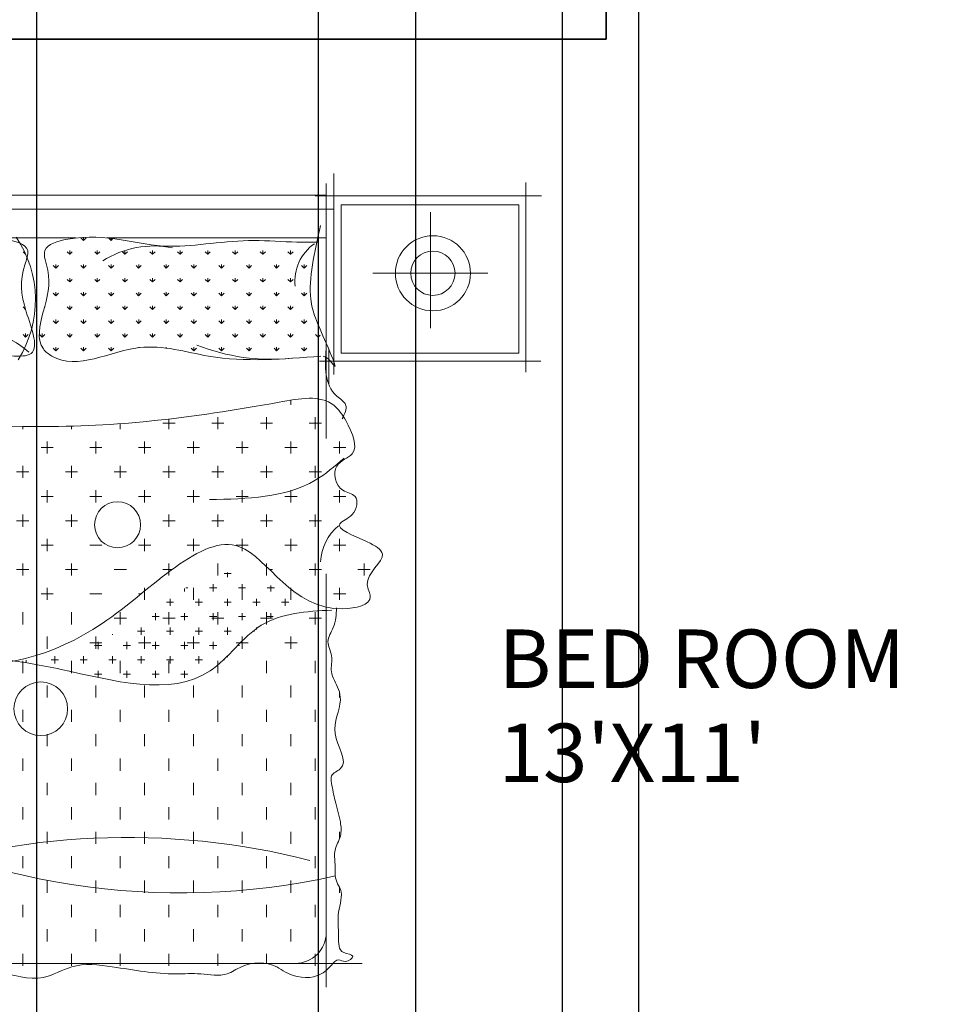
# Model space of a CAD drawing. Units: inches. Extents: x -438 to 102, y -60 to 1091.
# Tile 8 of 20: x -243 to -149, y 699 to 799. Entities that reach past the tile are written whole.
import ezdxf

# ---------------------------------------------------------------- set-up
doc = ezdxf.new("R2010")
doc.units = ezdxf.units.IN
doc.header["$MEASUREMENT"] = 0
doc.layers.add('A-ANNO-DIMS', color=217, linetype='Continuous', lineweight=18, true_color=0x93278f)
doc.layers.add('A-WALL', color=2, linetype='Continuous', lineweight=35, true_color=0xf1eb1f)
doc.layers.add('A-AREA-IDEN', color=4, linetype='Continuous', lineweight=18)
doc.layers.add('Furniture', color=7, linetype='Continuous', lineweight=15)
doc.styles.get("Standard").update_dxf_attribs({"font": 'arial.ttf'})
doc.dimstyles.get("Standard").update_dxf_attribs({"dimtxt": 8, "dimasz": 0.18, "dimexe": 0.18, "dimexo": 0.0625, "dimgap": 0.09, "dimtad": 0, "dimtih": 1, "dimtoh": 1, "dimdec": 4, "dimzin": 0, "dimdsep": 46, "dimlunit": 3, "dimtxsty": 'Standard', "dimcen": 0.09, "dimadec": 0, "dimazin": 0, "dimtfac": 1, "dimtdec": 4, "dimtofl": 0, "dimtmove": 0, "dimatfit": 3, "dimfxl": 1, "dimtolj": 1, "dimtzin": 0, "dimarcsym": 0})

# ---------------------------------------------------------------- blocks, each defined once
blk = doc.blocks.new('BED-DOUBLE-WITH-NIGHTSTANDS')
for p, q in [((30.68, 0), (30.68, -20.6)), ((50.37, -20.33), (50.37, -0.9)), ((29.9, -1.01), (29.9, -27.13)), ((-30.74, -2.19), (29.9, -2.19)), ((51.99, -2.28), (28.76, -2.28)), ((30.68, -3.64), (-30.92, -3.64)), ((49.65, -3.21), (31.43, -3.21)), ((31.43, -3.21), (31.43, -18.39)), ((40.58, -3.96), (40.58, -15.85)), ((49.65, -18.39), (49.65, -3.21)), ((4.24, -6.59), (-10.63, -6.59)), ((5.02, -6.85), (4.75, -6.59)), ((5.02, -6.85), (5.02, -6.53)), ((5.02, -6.85), (5.28, -6.59)), ((29.9, -6.59), (7.41, -6.59)), ((7.85, -6.85), (7.61, -6.61)), ((7.85, -6.85), (7.85, -6.64)), ((7.85, -6.85), (8.03, -6.66)), ((-0.92, -8.26), (-1.18, -8)), ((1.02, -8.02), (1.04, -8)), ((3.6, -8.26), (3.34, -8)), ((3.6, -8.27), (3.6, -7.89)), ((3.6, -8.26), (3.87, -8)), ((6.43, -8.26), (6.17, -8)), ((6.43, -8.27), (6.43, -7.89)), ((6.43, -8.26), (6.7, -8)), ((9.26, -8.26), (9, -8)), ((9.26, -8.27), (9.26, -7.89)), ((9.26, -8.26), (9.53, -8)), ((12.09, -8.26), (11.82, -8)), ((12.09, -8.27), (12.09, -7.89)), ((12.09, -8.26), (12.35, -8)), ((14.92, -8.26), (14.65, -8)), ((14.92, -8.27), (14.92, -7.89)), ((14.92, -8.26), (15.18, -8)), ((17.75, -8.26), (17.48, -8)), ((17.75, -8.27), (17.75, -7.89)), ((17.75, -8.26), (18.01, -8)), ((20.57, -8.26), (20.31, -8)), ((20.57, -8.27), (20.57, -7.89)), ((20.57, -8.26), (20.84, -8)), ((23.4, -8.26), (23.14, -8)), ((23.4, -8.27), (23.4, -7.89)), ((23.4, -8.26), (23.67, -8)), ((26.23, -8.26), (25.97, -8)), ((26.23, -8.27), (26.23, -7.89)), ((26.23, -8.26), (26.5, -8)), ((-0.92, -8.27), (-0.92, -8.26)), ((-0.92, -8.26), (-0.91, -8.26)), ((2.19, -9.68), (1.92, -9.41)), ((2.19, -9.68), (2.19, -9.3)), ((2.19, -9.68), (2.45, -9.41)), ((5.02, -9.68), (4.75, -9.41)), ((5.02, -9.68), (5.02, -9.3)), ((5.02, -9.68), (5.28, -9.41)), ((7.85, -9.68), (7.58, -9.41)), ((7.85, -9.68), (7.85, -9.3)), ((7.85, -9.68), (8.11, -9.41)), ((10.67, -9.68), (10.41, -9.41)), ((10.67, -9.68), (10.94, -9.41)), ((10.68, -9.68), (10.68, -9.3)), ((13.5, -9.68), (13.24, -9.41)), ((13.5, -9.68), (13.5, -9.3)), ((13.5, -9.68), (13.77, -9.41)), ((16.33, -9.68), (16.07, -9.41)), ((16.33, -9.68), (16.33, -9.3)), ((16.33, -9.68), (16.6, -9.41)), ((19.16, -9.68), (18.89, -9.41)), ((19.16, -9.68), (19.16, -9.3)), ((19.16, -9.68), (19.43, -9.41)), ((21.99, -9.68), (21.72, -9.41)), ((21.99, -9.68), (21.99, -9.3)), ((21.99, -9.68), (22.25, -9.41)), ((24.82, -9.68), (24.55, -9.41)), ((24.82, -9.68), (24.82, -9.3)), ((24.82, -9.68), (25.08, -9.41)), ((27.65, -9.68), (27.38, -9.41)), ((27.65, -9.68), (27.65, -9.3)), ((27.65, -9.68), (27.91, -9.41)), ((3.6, -11.09), (3.34, -10.83)), ((3.6, -11.09), (3.6, -10.72)), ((3.6, -11.09), (3.87, -10.83)), ((6.43, -11.09), (6.17, -10.83)), ((6.43, -11.09), (6.43, -10.72)), ((6.43, -11.09), (6.7, -10.83)), ((9.26, -11.09), (9, -10.83)), ((9.26, -11.09), (9.26, -10.72)), ((9.26, -11.09), (9.53, -10.83)), ((12.09, -11.09), (11.82, -10.83)), ((12.09, -11.09), (12.09, -10.72)), ((12.09, -11.09), (12.35, -10.83)), ((14.92, -11.09), (14.65, -10.83)), ((14.92, -11.09), (14.92, -10.72)), ((14.92, -11.09), (15.18, -10.83)), ((17.75, -11.09), (17.48, -10.83)), ((17.75, -11.09), (17.75, -10.72)), ((17.75, -11.09), (18.01, -10.83)), ((20.57, -11.09), (20.31, -10.83)), ((20.57, -11.09), (20.57, -10.72)), ((20.57, -11.09), (20.84, -10.83)), ((23.4, -11.09), (23.14, -10.83)), ((23.4, -11.09), (23.4, -10.72)), ((23.4, -11.09), (23.67, -10.83)), ((26.23, -11.09), (25.97, -10.83)), ((26.23, -11.09), (26.23, -10.72)), ((26.23, -11.09), (26.5, -10.83)), ((46.48, -10.21), (34.68, -10.21)), ((2.19, -12.51), (1.92, -12.24)), ((2.19, -12.51), (2.19, -12.13)), ((2.19, -12.51), (2.45, -12.24)), ((5.02, -12.51), (4.75, -12.24)), ((5.02, -12.51), (5.02, -12.13)), ((5.02, -12.51), (5.28, -12.24)), ((7.85, -12.51), (7.58, -12.24)), ((7.85, -12.51), (7.85, -12.13)), ((7.85, -12.51), (8.11, -12.24)), ((10.67, -12.51), (10.41, -12.24)), ((10.67, -12.51), (10.94, -12.24)), ((10.68, -12.51), (10.68, -12.13)), ((13.5, -12.51), (13.24, -12.24)), ((13.5, -12.51), (13.5, -12.13)), ((13.5, -12.51), (13.77, -12.24)), ((16.33, -12.51), (16.07, -12.24)), ((16.33, -12.51), (16.33, -12.13)), ((16.33, -12.51), (16.6, -12.24)), ((19.16, -12.51), (18.89, -12.24)), ((19.16, -12.51), (19.16, -12.13)), ((19.16, -12.51), (19.43, -12.24)), ((21.99, -12.51), (21.72, -12.24)), ((21.99, -12.51), (21.99, -12.13)), ((21.99, -12.51), (22.25, -12.24)), ((24.82, -12.51), (24.55, -12.24)), ((24.82, -12.51), (24.82, -12.13)), ((24.82, -12.51), (25.08, -12.24)), ((27.65, -12.51), (27.38, -12.24)), ((27.65, -12.51), (27.65, -12.13)), ((27.65, -12.51), (27.91, -12.24)), ((-0.93, -13.91), (-1.18, -13.66)), ((1.02, -13.67), (1.04, -13.66)), ((3.6, -13.92), (3.34, -13.66)), ((3.6, -13.92), (3.6, -13.55)), ((3.6, -13.92), (3.87, -13.66)), ((6.43, -13.92), (6.17, -13.66)), ((6.43, -13.92), (6.43, -13.55)), ((6.43, -13.92), (6.7, -13.66)), ((9.26, -13.92), (9, -13.66)), ((9.26, -13.92), (9.26, -13.55)), ((9.26, -13.92), (9.53, -13.66)), ((12.09, -13.92), (11.82, -13.66)), ((12.09, -13.92), (12.09, -13.55)), ((12.09, -13.92), (12.35, -13.66)), ((14.92, -13.92), (14.65, -13.66)), ((14.92, -13.92), (14.92, -13.55)), ((14.92, -13.92), (15.18, -13.66)), ((17.75, -13.92), (17.48, -13.66)), ((17.75, -13.92), (17.75, -13.55)), ((17.75, -13.92), (18.01, -13.66)), ((20.57, -13.92), (20.31, -13.66)), ((20.57, -13.92), (20.57, -13.55)), ((20.57, -13.92), (20.84, -13.66)), ((23.4, -13.92), (23.14, -13.66)), ((23.4, -13.92), (23.4, -13.55)), ((23.4, -13.92), (23.67, -13.66)), ((26.23, -13.92), (25.97, -13.66)), ((26.23, -13.92), (26.23, -13.55)), ((26.23, -13.92), (26.5, -13.66)), ((2.19, -15.34), (1.92, -15.07)), ((2.19, -15.34), (2.19, -14.96)), ((2.19, -15.34), (2.45, -15.07)), ((5.02, -15.34), (4.75, -15.07)), ((5.02, -15.34), (5.02, -14.96)), ((5.02, -15.34), (5.28, -15.07)), ((7.85, -15.34), (7.58, -15.07)), ((7.85, -15.34), (7.85, -14.96)), ((7.85, -15.34), (8.11, -15.07)), ((10.67, -15.34), (10.41, -15.07)), ((10.67, -15.34), (10.94, -15.07)), ((10.68, -15.34), (10.68, -14.96)), ((13.5, -15.34), (13.24, -15.07)), ((13.5, -15.34), (13.5, -14.96)), ((13.5, -15.34), (13.77, -15.07)), ((16.33, -15.34), (16.07, -15.07)), ((16.33, -15.34), (16.33, -14.96)), ((16.33, -15.34), (16.6, -15.07)), ((19.16, -15.34), (18.89, -15.07)), ((19.16, -15.34), (19.16, -14.96)), ((19.16, -15.34), (19.43, -15.07)), ((21.99, -15.34), (21.72, -15.07)), ((21.99, -15.34), (21.99, -14.96)), ((21.99, -15.34), (22.25, -15.07)), ((24.82, -15.34), (24.55, -15.07)), ((24.82, -15.34), (24.82, -14.96)), ((24.82, -15.34), (25.08, -15.07)), ((27.65, -15.34), (27.38, -15.07)), ((27.65, -15.34), (27.65, -14.96)), ((27.65, -15.34), (27.91, -15.07)), ((-0.92, -16.75), (-1.18, -16.48)), ((-0.92, -16.75), (-0.92, -16.38)), ((-0.92, -16.75), (-0.65, -16.48)), ((0.78, -16.75), (0.51, -16.48)), ((0.78, -16.75), (0.78, -16.38)), ((0.78, -16.75), (1.04, -16.48)), ((3.6, -16.75), (3.34, -16.48)), ((3.6, -16.75), (3.6, -16.38)), ((3.6, -16.75), (3.87, -16.48)), ((6.43, -16.75), (6.17, -16.48)), ((6.43, -16.75), (6.43, -16.38)), ((6.43, -16.75), (6.7, -16.48)), ((9.26, -16.75), (9, -16.48)), ((9.26, -16.75), (9.26, -16.38)), ((9.26, -16.75), (9.53, -16.48)), ((12.09, -16.75), (11.82, -16.48)), ((12.09, -16.75), (12.09, -16.38)), ((12.09, -16.75), (12.35, -16.48)), ((14.92, -16.75), (14.65, -16.48)), ((14.92, -16.75), (14.92, -16.38)), ((14.92, -16.75), (15.18, -16.48)), ((17.75, -16.75), (17.48, -16.48)), ((17.75, -16.75), (17.75, -16.38)), ((17.75, -16.75), (18.01, -16.48)), ((20.57, -16.75), (20.31, -16.48)), ((20.57, -16.75), (20.57, -16.38)), ((20.57, -16.75), (20.84, -16.48)), ((23.4, -16.75), (23.14, -16.48)), ((23.4, -16.75), (23.4, -16.38)), ((23.4, -16.75), (23.67, -16.48)), ((26.23, -16.75), (25.97, -16.48)), ((26.23, -16.75), (26.23, -16.38)), ((26.23, -16.75), (26.5, -16.48)), ((29.06, -16.75), (28.79, -16.48)), ((29.06, -16.75), (29.06, -16.38)), ((29.06, -16.75), (29.27, -16.54)), ((2.19, -18.16), (1.92, -17.9)), ((2.19, -18.16), (2.19, -17.79)), ((2.19, -18.16), (2.45, -17.9)), ((5.02, -18.16), (4.75, -17.9)), ((5.02, -18.16), (5.02, -17.79)), ((5.02, -18.16), (5.28, -17.9)), ((7.85, -18.16), (7.58, -17.9)), ((7.85, -18.16), (7.85, -17.79)), ((7.85, -18.16), (8.11, -17.9)), ((10.68, -17.83), (10.68, -17.79)), ((13.5, -17.88), (13.5, -17.79)), ((13.76, -17.91), (13.77, -17.9)), ((16.33, -18.16), (16.07, -17.9)), ((16.33, -18.16), (16.33, -17.79)), ((16.33, -18.16), (16.6, -17.9)), ((19.16, -18.16), (18.89, -17.9)), ((19.16, -18.16), (19.16, -17.79)), ((19.16, -18.16), (19.43, -17.9)), ((21.99, -18.16), (21.72, -17.9)), ((21.99, -18.16), (21.99, -17.79)), ((21.99, -18.16), (22.25, -17.9)), ((24.82, -18.16), (24.55, -17.9)), ((24.82, -18.16), (24.82, -17.79)), ((24.82, -18.16), (25.08, -17.9)), ((27.65, -18.16), (27.38, -17.9)), ((27.65, -18.16), (27.65, -17.79)), ((27.65, -18.16), (27.91, -17.9)), ((30.17, -21.62), (30.17, -17.94)), ((31.43, -18.39), (49.65, -18.39)), ((3.6, -19.24), (3.6, -19.2)), ((29.21, -19.21), (51.9, -19.21)), ((26.28, -23.69), (26.28, -23.21)), ((13.78, -26.19), (13.78, -25.14)), ((18.78, -26.19), (18.78, -24.94)), ((23.78, -26.19), (23.78, -24.94)), ((28.78, -26.19), (28.78, -24.94)), ((-1.22, -26.19), (-1.22, -25.9)), ((3.78, -26.19), (3.78, -25.87)), ((8.78, -26.19), (8.78, -25.62)), ((14.41, -25.57), (13.16, -25.57)), ((19.41, -25.57), (18.16, -25.57)), ((24.41, -25.57), (23.16, -25.57)), ((29.41, -25.57), (28.16, -25.57)), ((1.91, -28.07), (0.66, -28.07)), ((1.28, -28.69), (1.28, -27.44)), ((6.91, -28.07), (5.66, -28.07)), ((6.28, -28.69), (6.28, -27.44)), ((11.91, -28.07), (10.66, -28.07)), ((11.28, -28.69), (11.28, -27.44)), ((16.91, -28.07), (15.66, -28.07)), ((16.28, -28.69), (16.28, -27.44)), ((21.91, -28.07), (20.66, -28.07)), ((21.28, -28.69), (21.28, -27.44)), ((26.91, -28.07), (25.66, -28.07)), ((26.28, -28.69), (26.28, -27.44)), ((31.91, -28.07), (30.66, -28.07)), ((31.28, -28.69), (31.28, -27.44)), ((-1.22, -31.19), (-1.22, -29.94)), ((3.78, -31.19), (3.78, -29.94)), ((8.78, -31.19), (8.78, -29.94)), ((13.78, -31.19), (13.78, -29.94)), ((18.78, -31.19), (18.78, -29.94)), ((23.78, -31.19), (23.78, -29.94)), ((28.78, -31.19), (28.78, -29.94)), ((-0.59, -30.57), (-1.84, -30.57)), ((4.41, -30.57), (3.16, -30.57)), ((9.41, -30.57), (8.16, -30.57)), ((14.41, -30.57), (13.16, -30.57)), ((19.41, -30.57), (18.16, -30.57)), ((24.41, -30.57), (23.16, -30.57)), ((29.41, -30.57), (28.16, -30.57)), ((1.91, -33.07), (0.66, -33.07)), ((1.28, -33.69), (1.28, -32.44)), ((6.91, -33.07), (5.66, -33.07)), ((6.28, -33.69), (6.28, -32.44)), ((11.91, -33.07), (10.66, -33.07)), ((11.28, -33.69), (11.28, -32.44)), ((16.91, -33.07), (15.66, -33.07)), ((16.28, -33.69), (16.28, -32.44)), ((21.91, -33.07), (20.66, -33.07)), ((21.28, -33.69), (21.28, -32.44)), ((26.91, -33.07), (25.66, -33.07)), ((26.28, -33.69), (26.28, -32.44)), ((31.91, -33.07), (30.66, -33.07)), ((31.28, -33.69), (31.28, -32.44)), ((-1.22, -36.19), (-1.22, -34.94)), ((3.78, -36.19), (3.78, -34.94)), ((13.78, -36.19), (13.78, -34.94)), ((18.78, -36.19), (18.78, -34.94)), ((23.78, -36.19), (23.78, -34.94)), ((28.78, -36.19), (28.78, -34.94)), ((-0.59, -35.57), (-1.84, -35.57)), ((4.41, -35.57), (3.16, -35.57)), ((14.41, -35.57), (13.16, -35.57)), ((19.41, -35.57), (18.16, -35.57)), ((24.41, -35.57), (23.16, -35.57)), ((29.41, -35.57), (28.16, -35.57)), ((1.91, -38.07), (0.66, -38.07)), ((1.28, -38.69), (1.28, -37.44)), ((6.91, -38.07), (5.66, -38.07)), ((11.91, -38.07), (10.66, -38.07)), ((11.28, -38.69), (11.28, -37.44)), ((16.91, -38.07), (15.66, -38.07)), ((16.28, -38.69), (16.28, -37.44)), ((21.91, -38.07), (20.66, -38.07)), ((21.28, -38.69), (21.28, -37.44)), ((26.91, -38.07), (25.66, -38.07)), ((26.28, -38.69), (26.28, -37.44)), ((31.91, -38.07), (30.66, -38.07)), ((31.28, -38.69), (31.28, -37.44)), ((-1.22, -41.19), (-1.22, -39.94)), ((3.78, -41.19), (3.78, -39.94)), ((13.78, -41.19), (13.78, -39.94)), ((18.78, -41.19), (18.78, -39.94)), ((23.78, -41.19), (23.78, -39.94)), ((28.78, -41.19), (28.78, -39.94)), ((33.78, -41.19), (33.78, -39.94)), ((-0.59, -40.57), (-1.84, -40.57)), ((4.41, -40.57), (3.16, -40.57)), ((9.41, -40.57), (8.16, -40.57)), ((14.1, -40.57), (13.16, -40.57)), ((20.16, -40.97), (19.43, -40.97)), ((19.79, -41.34), (19.79, -40.86)), ((24.41, -40.57), (24.09, -40.57)), ((29.41, -40.57), (28.16, -40.57)), ((29.9, -41), (29.9, -83.36)), ((34.41, -40.57), (33.16, -40.57)), ((18.32, -42.82), (18.32, -42.08)), ((21.27, -42.82), (21.27, -42.08)), ((24.22, -42.82), (24.22, -42.22)), ((1.91, -43.07), (0.66, -43.07)), ((1.28, -43.69), (1.28, -42.44)), ((6.91, -43.07), (5.66, -43.07)), ((10.92, -43.07), (10.66, -43.07)), ((11.28, -43.69), (11.28, -42.44)), ((15.37, -42.82), (15.37, -42.52)), ((15.73, -42.45), (15.5, -42.45)), ((16.28, -43.69), (16.28, -42.44)), ((18.69, -42.45), (17.95, -42.45)), ((21.64, -42.45), (20.9, -42.45)), ((21.28, -43.69), (21.28, -42.44)), ((24.59, -42.45), (23.85, -42.45)), ((26.28, -43.69), (26.28, -42.44)), ((31.91, -43.07), (30.66, -43.07)), ((31.28, -43.69), (31.28, -42.44)), ((14.26, -43.92), (13.52, -43.92)), ((13.89, -44.29), (13.89, -43.56)), ((17.21, -43.92), (16.47, -43.92)), ((16.84, -44.29), (16.84, -43.56)), ((20.16, -43.92), (19.43, -43.92)), ((19.79, -44.29), (19.79, -43.56)), ((23.12, -43.92), (22.38, -43.92)), ((22.75, -44.29), (22.75, -43.56)), ((26.07, -43.92), (25.33, -43.92)), ((25.7, -44.29), (25.7, -43.56)), ((-1.22, -46.19), (-1.22, -44.94)), ((3.78, -46.19), (3.78, -44.94)), ((8.78, -46.19), (8.78, -44.94)), ((12.78, -45.4), (12.04, -45.4)), ((12.41, -45.77), (12.41, -45.03)), ((13.78, -46.19), (13.78, -44.94)), ((15.73, -45.4), (15, -45.4)), ((15.37, -45.77), (15.37, -45.03)), ((18.69, -45.4), (17.95, -45.4)), ((18.32, -45.77), (18.32, -45.03)), ((18.78, -46.19), (18.78, -44.94)), ((21.64, -45.4), (20.9, -45.4)), ((21.27, -45.77), (21.27, -45.03)), ((23.78, -46.19), (23.78, -44.94)), ((24.47, -45.4), (23.85, -45.4)), ((24.22, -45.56), (24.22, -45.03)), ((28.78, -46.19), (28.78, -44.94)), ((9.41, -45.57), (8.16, -45.57)), ((14.41, -45.57), (13.16, -45.57)), ((19.41, -45.57), (18.16, -45.57)), ((24.41, -45.57), (23.16, -45.57)), ((29.41, -45.57), (28.16, -45.57)), ((7.98, -47.25), (7.98, -47.2)), ((11.31, -46.88), (10.57, -46.88)), ((10.94, -47.25), (10.94, -46.51)), ((14.26, -46.88), (13.52, -46.88)), ((13.89, -47.25), (13.89, -46.51)), ((17.21, -46.88), (16.47, -46.88)), ((16.84, -47.25), (16.84, -46.51)), ((20.16, -46.88), (19.43, -46.88)), ((19.79, -47.25), (19.79, -46.51)), ((22.55, -46.88), (22.38, -46.88)), ((22.75, -46.7), (22.75, -46.51)), ((1.28, -48.69), (1.28, -47.44)), ((6.91, -48.07), (5.66, -48.07)), ((6.88, -48.35), (6.14, -48.35)), ((6.28, -48.69), (6.28, -47.44)), ((6.51, -48.72), (6.51, -47.98)), ((9.83, -48.35), (9.09, -48.35)), ((9.46, -48.72), (9.46, -47.98)), ((11.91, -48.07), (10.66, -48.07)), ((11.28, -48.69), (11.28, -47.44)), ((12.78, -48.35), (12.04, -48.35)), ((12.41, -48.72), (12.41, -47.98)), ((15.73, -48.35), (15, -48.35)), ((15.37, -48.72), (15.37, -47.98)), ((16.91, -48.07), (15.66, -48.07)), ((16.28, -48.69), (16.28, -47.44)), ((18.69, -48.35), (17.95, -48.35)), ((18.32, -48.72), (18.32, -47.98)), ((21.91, -48.07), (20.66, -48.07)), ((21.02, -48.35), (20.9, -48.35)), ((21.27, -48.11), (21.27, -47.98)), ((21.28, -48.69), (21.28, -47.44)), ((26.91, -48.07), (25.66, -48.07)), ((26.28, -48.69), (26.28, -47.44)), ((-1.22, -51.19), (-1.22, -49.94)), ((-0.87, -50.11), (-0.87, -49.87)), ((2.45, -49.83), (1.71, -49.83)), ((2.08, -50.2), (2.08, -49.46)), ((3.78, -51.19), (3.78, -49.94)), ((5.4, -49.83), (4.66, -49.83)), ((5.03, -50.2), (5.03, -49.46)), ((8.35, -49.83), (7.61, -49.83)), ((7.98, -50.2), (7.98, -49.46)), ((8.78, -51.19), (8.78, -49.94)), ((11.31, -49.83), (10.57, -49.83)), ((10.94, -50.2), (10.94, -49.46)), ((14.26, -49.83), (13.52, -49.83)), ((13.78, -51.19), (13.78, -49.94)), ((13.89, -50.2), (13.89, -49.46)), ((17.21, -49.83), (16.47, -49.83)), ((16.84, -50.2), (16.84, -49.46)), ((18.78, -51.19), (18.78, -49.94)), ((19.48, -49.83), (19.43, -49.83)), ((19.79, -49.55), (19.79, -49.46)), ((23.78, -51.19), (23.78, -49.94)), ((28.78, -51.19), (28.78, -49.94)), ((3.55, -50.99), (3.55, -50.94)), ((6.88, -51.31), (6.14, -51.31)), ((6.51, -51.61), (6.51, -50.94)), ((9.83, -51.31), (9.09, -51.31)), ((9.46, -51.68), (9.46, -50.94)), ((12.78, -51.31), (12.04, -51.31)), ((12.41, -51.68), (12.41, -50.94)), ((15.73, -51.31), (15, -51.31)), ((15.37, -51.68), (15.37, -50.94)), ((1.28, -53.69), (1.28, -52.44)), ((6.28, -53.69), (6.28, -52.44)), ((11.28, -53.69), (11.28, -52.44)), ((16.28, -53.69), (16.28, -52.44)), ((21.28, -53.69), (21.28, -52.44)), ((26.28, -53.69), (26.28, -52.44)), ((31.28, -53.69), (31.28, -53.25)), ((-1.22, -56.19), (-1.22, -54.94)), ((3.78, -56.19), (3.78, -54.94)), ((8.78, -56.19), (8.78, -54.94)), ((13.78, -56.19), (13.78, -54.94)), ((18.78, -56.19), (18.78, -54.94)), ((23.78, -56.19), (23.78, -54.94)), ((28.78, -56.19), (28.78, -54.94)), ((1.28, -58.69), (1.28, -57.44)), ((6.28, -58.69), (6.28, -57.44)), ((11.28, -58.69), (11.28, -57.44)), ((16.28, -58.69), (16.28, -57.44)), ((21.28, -58.69), (21.28, -57.44)), ((26.28, -58.69), (26.28, -57.44)), ((-1.22, -61.19), (-1.22, -59.94)), ((3.78, -61.19), (3.78, -59.94)), ((8.78, -61.19), (8.78, -59.94)), ((13.78, -61.19), (13.78, -59.94)), ((18.78, -61.19), (18.78, -59.94)), ((23.78, -61.19), (23.78, -59.94)), ((28.78, -61.19), (28.78, -59.94)), ((1.28, -63.69), (1.28, -62.44)), ((6.28, -63.69), (6.28, -62.44)), ((11.28, -63.69), (11.28, -62.44)), ((16.28, -63.69), (16.28, -62.44)), ((21.28, -63.69), (21.28, -62.44)), ((26.28, -63.69), (26.28, -62.44)), ((-1.22, -66.19), (-1.22, -64.94)), ((3.78, -66.19), (3.78, -64.94)), ((8.78, -66.19), (8.78, -64.94)), ((13.78, -66.19), (13.78, -64.94)), ((18.78, -66.19), (18.78, -64.94)), ((23.78, -66.19), (23.78, -64.94)), ((28.78, -66.19), (28.78, -64.94)), ((1.28, -68.69), (1.28, -67.44)), ((6.28, -68.69), (6.28, -67.44)), ((11.28, -68.69), (11.28, -67.44)), ((16.28, -68.69), (16.28, -67.44)), ((21.28, -68.69), (21.28, -67.44)), ((26.28, -68.69), (26.28, -67.44)), ((31.28, -68.1), (31.28, -67.44)), ((-1.22, -71.19), (-1.22, -69.94)), ((3.78, -71.19), (3.78, -69.94)), ((8.78, -71.19), (8.78, -69.94)), ((13.78, -71.19), (13.78, -69.94)), ((18.78, -71.19), (18.78, -69.94)), ((23.78, -71.19), (23.78, -69.94)), ((28.78, -71.19), (28.78, -69.94)), ((1.28, -73.69), (1.28, -72.44)), ((6.28, -73.69), (6.28, -72.44)), ((11.28, -73.69), (11.28, -72.44)), ((16.28, -73.69), (16.28, -72.44)), ((21.28, -73.69), (21.28, -72.44)), ((26.28, -73.69), (26.28, -72.44)), ((31.28, -73.69), (31.28, -73.16)), ((-1.22, -76.19), (-1.22, -74.94)), ((3.78, -76.19), (3.78, -74.94)), ((8.78, -76.19), (8.78, -74.94)), ((13.78, -76.19), (13.78, -74.94)), ((18.78, -76.19), (18.78, -74.94)), ((23.78, -76.19), (23.78, -74.94)), ((28.78, -76.19), (28.78, -74.94)), ((1.28, -78.69), (1.28, -77.44)), ((6.28, -78.69), (6.28, -77.44)), ((11.28, -78.69), (11.28, -77.44)), ((16.28, -78.69), (16.28, -77.44)), ((21.28, -78.69), (21.28, -77.44)), ((26.28, -78.69), (26.28, -77.44)), ((-1.22, -81.19), (-1.22, -79.94)), ((3.78, -81.19), (3.78, -79.94)), ((8.78, -81.19), (8.78, -79.94)), ((13.78, -81.19), (13.78, -79.94)), ((18.78, -81.19), (18.78, -79.94)), ((23.78, -80.94), (23.78, -79.94)), ((28.78, -81.19), (28.78, -79.94)), ((33.6, -80.93), (-28.29, -80.93))]:
    blk.add_line(p, q)
for centre, radius in [((40.84, -10.21), 3.85), ((40.84, -10.21), 2.27), ((8.51, -35.98), 2.36), ((0.64, -54.84), 2.75)]:
    blk.add_circle(centre, radius)
for centre, radius, start, end in [((-11.37, -12.95), 11.46, 327.7555, 34.1397), ((12.25, -17.2), 9.79, 78.7884, 122.5362), ((31.35, -11.01), 4.66, 124.7345, 186.5526), ((-7.57, -26.26), 10.59, 48.8713, 93.3448), ((24.21, 1.34), 20.36, 248.1857, 275.9106), ((34.27, -39.94), 4.94, 128.8354, 178.0038), ((14.99, -0.75), 72.97, 239.8126, 282.5472), ((9.5, -143.88), 75.85, 75.7143, 109.4459), ((26.75, -77.78), 3.15, 270, 0)]:
    blk.add_arc(centre, radius, start, end)
for points, knots in [([(-27.27, -18.7), (-25.92, -18.73), (-18.98, -18.88), (-10.03, -16.15), (-2.96, -18.87), (0.8, -18.49), (-1.35, -13.48), (-1.55, -10.6), (-0.23, -7.33), (-8.54, -5.31), (-15.4, -8.29), (-23.67, -6.97), (-26.61, -7), (-27.15, -7.01)], [0, 0, 0, 0, 4.049674, 20.880819, 25.932041, 26.821979, 31.217024, 36.043065, 37.533831, 40.150607, 55.448466, 62.672935, 64.278467, 64.278467, 64.278467, 64.278467]), ([(29.35, -18.7), (25.48, -19.02), (19.22, -19.53), (10.28, -16.58), (3.99, -20.47), (0.06, -17.44), (0.95, -13.79), (1.87, -10.79), (0.46, -7.43), (6.72, -5.67), (11.66, -7.91), (18.15, -7.12), (22.47, -6.73), (26.14, -7.04), (28.33, -7.01), (29.06, -7.01)], [0, 0, 0, 0, 11.502554, 18.635017, 27.654655, 28.800011, 32.595859, 36.914018, 38.927328, 41.544104, 52.009639, 56.262652, 60.661637, 65.075538, 67.252844, 67.252844, 67.252844, 67.252844]), ([(29.32, -5.32), (28.7, -8.05), (27.69, -12.51), (29.2, -15.74), (31.39, -20.84), (30.11, -18.79), (29.6, -18.7)], [0, 0, 0, 0, 7.603099, 12.404488, 14.892294, 16.432626, 16.432626, 16.432626, 16.432626]), ([(29.9, -17.94), (29.78, -19.78), (29.64, -22.09), (32.27, -23.65), (31.79, -24.62), (31.53, -25.14)], [0, 0, 0, 0, 4.973031, 6.254082, 7.747585, 7.747585, 7.747585, 7.747585]), ([(31.93, -25.29), (32.57, -26.62), (33.59, -28.72), (30.29, -29.71), (31.01, -32.64), (33.35, -32.83), (32.92, -35.12), (30.08, -36.11), (33.79, -37.48), (36.78, -39.18), (33.39, -41.32), (35.07, -44.06), (26.87, -46.02), (20.99, -32.35), (2.1, -54.12), (-16.08, -50.43), (-31.16, -41.37), (-34.82, -50.79), (-35.75, -45.56), (-33.27, -44.57), (-36.07, -39.92), (-29.61, -39.91), (-31.05, -37.18), (-31.79, -35.41), (-31.67, -30.43), (-16.86, -30.76), (-35.73, -24.41), (-25.68, -23.88), (-16.82, -24.97), (2.34, -26.69), (17.46, -24.9), (30.09, -22.48), (31.54, -24.71), (31.93, -25.29)], [0, 0, 0, 0, 3.481099, 5.475811, 8.043407, 9.436812, 11.330727, 12.888379, 16.258255, 18.252967, 21.734596, 23.018392, 26.087149, 38.445812, 54.5649, 86.600283, 92.594507, 98.286547, 100.905288, 101.70342, 105.471876, 109.954916, 110.954151, 113.598333, 116.114301, 124.231953, 133.25029, 137.509046, 143.991555, 164.906349, 189.961005, 195.579007, 197.573325, 197.573325, 197.573325, 197.573325]), ([(31.74, -29.16), (30.78, -29.98), (26.99, -33.22), (21.81, -33.32), (17.94, -33.4)], [0, 0, 0, 0, 3.737027, 14.742384, 14.742384, 14.742384, 14.742384]), ([(30.96, -44.51), (30.93, -45.19), (30.86, -46.38), (29.77, -47.93), (30.68, -49.44), (30.18, -51.19), (31.18, -52.55), (31.56, -54.75), (29.86, -57.22), (32.61, -60.74), (30.28, -61.5), (30.52, -62.88), (30.79, -64.38), (31.38, -66.15), (31.51, -67.95), (30.62, -69.27), (30.89, -70.9), (30.72, -72.32), (31.74, -73.74), (30.93, -75.81), (31.25, -77.78), (31.09, -79.97), (33.09, -80.01), (31.89, -81), (31.1, -80.32), (30.21, -81.43), (28.73, -82.66), (26.29, -82.31), (24.17, -80.73), (21.7, -80.78), (19.49, -82.4), (17.06, -81.88), (13.17, -82.17), (8.82, -81.36), (4.07, -80.77), (0.46, -83.09), (-2.79, -81.85), (-5.87, -81.65), (-14.3, -79.69), (-20.14, -80.18), (-31.55, -83.45), (-29.78, -79.6), (-32.81, -83.8), (-29.07, -82.96), (-24.85, -82.73), (-30.36, -81.5), (-32.31, -79.09), (-32.11, -72.2), (-27.72, -79.52), (-31.69, -72.6), (-28.72, -70.51), (-27.65, -65.93), (-35.2, -65.77), (-26.02, -64.12), (-35.79, -62.68), (-27.32, -61.35), (-31.95, -58.4), (-27.39, -55.21), (-31.95, -53.76), (-28.5, -51.75), (-29.55, -48.81), (-29.07, -42.18), (-29.13, -46.29), (-29.16, -48.01)], [0, 0, 0, 0, 2.033881, 3.581387, 5.07489, 6.704853, 8.655612, 9.757262, 13.24098, 16.903694, 18.063816, 18.788243, 20.635227, 22.875483, 24.324336, 25.871843, 27.320698, 29.140811, 29.950855, 32.312207, 34.847704, 36.565952, 37.541804, 38.447727, 39.194923, 40.100844, 41.912688, 45.194843, 46.251388, 49.875946, 51.496686, 54.215105, 56.7523, 63.316606, 67.484853, 70.581422, 75.324573, 76.965649, 79.915763, 100.671038, 102.483321, 104.317501, 106.523635, 109.038061, 111.571263, 115.809372, 117.667229, 122.411431, 125.445794, 129.976907, 132.758854, 136.424739, 139.918708, 143.481583, 147.135325, 151.002466, 153.252794, 157.23352, 159.244583, 161.905351, 164.097269, 169.015093, 172.531686, 172.531686, 172.531686, 172.531686]), ([(30.47, -44.73), (27.88, -44.87), (22.83, -45.15), (16.72, -54.5), (5.64, -51.25), (-8.89, -48.66), (-19.85, -50.38), (-33.1, -52.54), (-34.5, -49.21), (-35, -48.01)], [0, 0, 0, 0, 7.385187, 14.402621, 29.694422, 35.583277, 59.348121, 65.733553, 69.320983, 69.320983, 69.320983, 69.320983])]:
    blk.add_open_spline(points, degree=3, knots=knots)
blk = doc.blocks.new('*D37')
at = {"layer": 'A-ANNO-DIMS', "color": 0, "lineweight": -2, "transparency": 16777216}
for p, q in [((-179.8, 234.94), (-179.8, 1079.58)), ((-179.62, 1079.4), (-176.98, 1079.4)), ((-134.26, 1079.4), (-136.9, 1079.4)), ((-134.08, 234.94), (-134.08, 1079.58))]:
    blk.add_line(p, q, dxfattribs=at)
at = {"layer": 'A-ANNO-DIMS', "color": 0, "transparency": 16777216}
for points in [[(-179.62, 1079.43), (-179.62, 1079.37), (-179.8, 1079.4)], [(-134.26, 1079.43), (-134.26, 1079.37), (-134.08, 1079.4)]]:
    blk.add_solid(points, dxfattribs=at)
at = {"layer": 'Defpoints', "color": 0, "transparency": 16777216}
for p in [(-134.08, 1079.4), (-179.8, 234.88), (-134.08, 234.88)]:
    blk.add_point(p, dxfattribs=at)
at = {"layer": 'A-ANNO-DIMS', "color": 0, "transparency": 16777216, "insert": (-156.94, 1079.4), "char_height": 8, "attachment_point": 5}
blk.add_mtext('\\A1;3\'-9 1/2"', dxfattribs=at)
blk = doc.blocks.new('*D51')
at = {"layer": 'A-ANNO-DIMS', "color": 0, "lineweight": -2, "transparency": 16777216}
for p, q in [((-291.54, 847), (-291.54, -48.58)), ((-275.79, 847), (-275.79, -48.58)), ((-291.36, -48.4), (-275.97, -48.4)), ((-275.79, -48.4), (-275.61, -48.4))]:
    blk.add_line(p, q, dxfattribs=at)
at = {"layer": 'A-ANNO-DIMS', "color": 0, "transparency": 16777216}
for points in [[(-291.36, -48.37), (-291.36, -48.43), (-291.54, -48.4)], [(-275.97, -48.37), (-275.97, -48.43), (-275.79, -48.4)]]:
    blk.add_solid(points, dxfattribs=at)
at = {"layer": 'Defpoints', "color": 0, "transparency": 16777216}
for p in [(-291.54, 847.06), (-275.79, 847.06), (-275.79, -48.4)]:
    blk.add_point(p, dxfattribs=at)
at = {"layer": 'A-ANNO-DIMS', "color": 0, "transparency": 16777216, "insert": (-255.95, -48.4), "char_height": 8, "attachment_point": 5}
blk.add_mtext('\\A1;1\'-3 1/2"', dxfattribs=at)
blk = doc.blocks.new('*D55')
at = {"layer": 'A-ANNO-DIMS', "color": 0, "lineweight": -2, "transparency": 16777216}
for p, q in [((-241.57, 808.32), (-241.57, -48.58)), ((-187.65, 801.94), (-187.65, -48.58)), ((-241.39, -48.4), (-225.49, -48.4)), ((-187.83, -48.4), (-203.72, -48.4))]:
    blk.add_line(p, q, dxfattribs=at)
at = {"layer": 'A-ANNO-DIMS', "color": 0, "transparency": 16777216}
for points in [[(-241.39, -48.37), (-241.39, -48.43), (-241.57, -48.4)], [(-187.83, -48.37), (-187.83, -48.43), (-187.65, -48.4)]]:
    blk.add_solid(points, dxfattribs=at)
at = {"layer": 'Defpoints', "color": 0, "transparency": 16777216}
for p in [(-241.57, 808.38), (-187.65, 802), (-187.65, -48.4)]:
    blk.add_point(p, dxfattribs=at)
at = {"layer": 'A-ANNO-DIMS', "color": 0, "transparency": 16777216, "insert": (-214.61, -48.4), "char_height": 8, "attachment_point": 5}
blk.add_mtext('\\A1;4\'-6"', dxfattribs=at)
blk = doc.blocks.new('*D61')
at = {"layer": 'A-ANNO-DIMS', "color": 0, "lineweight": -2, "transparency": 16777216}
for p, q in [((-212.65, 1079.4), (-212.83, 1079.4)), ((-212.65, 534.56), (-212.65, 1079.58)), ((-202.83, 1079.4), (-212.47, 1079.4)), ((-202.65, 534.56), (-202.65, 1079.58))]:
    blk.add_line(p, q, dxfattribs=at)
at = {"layer": 'A-ANNO-DIMS', "color": 0, "transparency": 16777216}
for points in [[(-212.47, 1079.43), (-212.47, 1079.37), (-212.65, 1079.4)], [(-202.83, 1079.43), (-202.83, 1079.37), (-202.65, 1079.4)]]:
    blk.add_solid(points, dxfattribs=at)
at = {"layer": 'Defpoints', "color": 0, "transparency": 16777216}
for p in [(-212.65, 1079.4), (-212.65, 534.5), (-202.65, 534.5)]:
    blk.add_point(p, dxfattribs=at)
at = {"layer": 'A-ANNO-DIMS', "color": 0, "transparency": 16777216, "insert": (-226.66, 1079.4), "char_height": 8, "attachment_point": 5}
blk.add_mtext('\\A1;0\'-10"', dxfattribs=at)

msp = doc.modelspace()

# ---------------------------------------------------------------- linework, layer by layer
at = {"layer": 'A-WALL'}
for p, q in [((-183.14649, 839.49939), (-183.14649, 797.49939)), ((-183.14649, 797.49939), (-303.14649, 797.49939))]:
    msp.add_line(p, q, dxfattribs=at)

# ---------------------------------------------------------------- block references
at = {"layer": 'Furniture'}
msp.add_blockref('BED-DOUBLE-WITH-NIGHTSTANDS', (-241.75124, 783.71416), dxfattribs=at)

# ---------------------------------------------------------------- texts
at = {"layer": 'A-AREA-IDEN'}
for s, p in [('BED ROOM', (-194.15703, 730.99783)), ("13'X11'", (-194.15703, 721.35935))]:
    msp.add_text(s, height=6, dxfattribs=at).set_placement(p)

# ---------------------------------------------------------------- dimensions: what is measured, and where the dimension line sits
at = {"layer": 'A-ANNO-DIMS'}
for base, p1, p2, picture, middle in [((-134.07948, 1079.39939), (-179.79585, 234.87846), (-134.07948, 234.87846), '*D37', (-156.93767, 1079.39939)), ((-212.64649, 1079.39939), (-202.64649, 534.49939), (-212.64649, 534.49939), '*D61', (-226.65728, 1079.39939)), ((-275.79225, -48.40061), (-291.54025, 847.06395), (-275.79225, 847.06395), '*D51', (-255.94517, -48.40061)), ((-187.64649, -48.40061), (-241.57044, 808.38394), (-187.64649, 801.99939), '*D55', (-214.60846, -48.40061))]:
    dim = msp.add_linear_dim(base=base, p1=p1, p2=p2, dimstyle='Standard', override={"dimdec": 1, "dimlfac": 1, "dimrnd": 0, "dimzin": 1, "dimdsep": 46, "dimlunit": 4, "dimfrac": 2}, dxfattribs=at)
    dim.commit()
    dim.dimension.update_dxf_attribs({"geometry": picture, "text_midpoint": middle})

doc.saveas('drawing.dxf')
